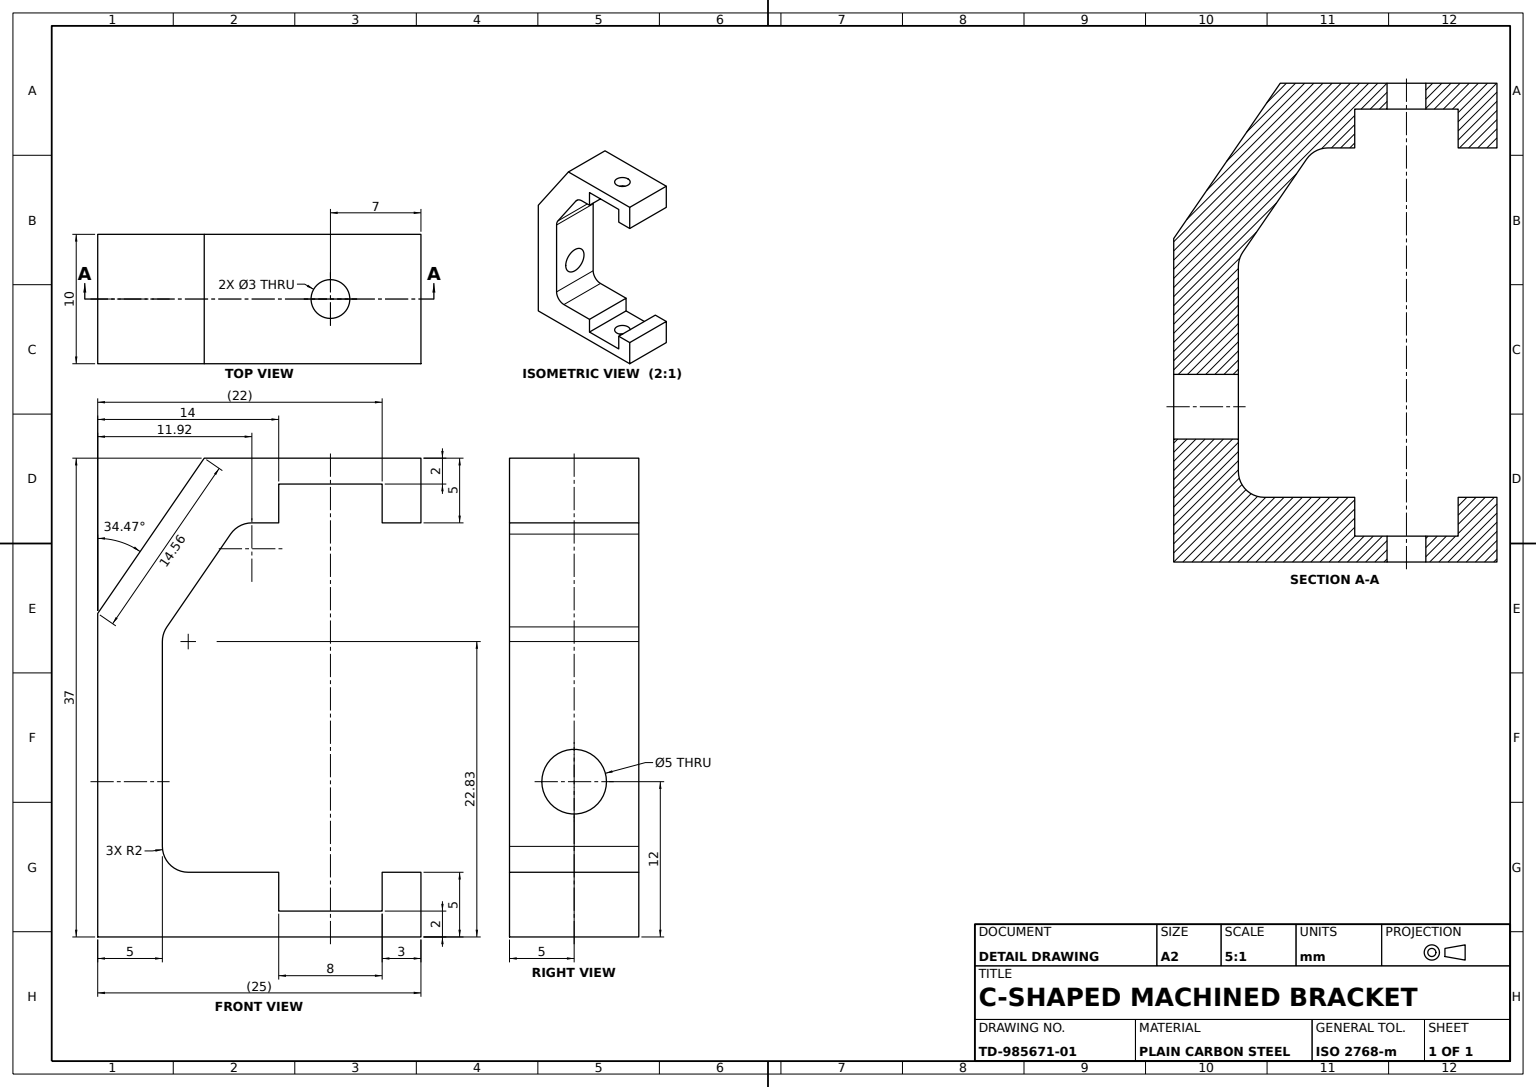
SolidWorks part; units mm, degrees
material "Plain Carbon Steel"
ref_plane "Front Plane" through (0, 0, 0) normal (0, 0, 1) x (1, 0, 0)
ref_plane "Top Plane" through (0, 0, 0) normal (0, 1, 0) x (1, 0, 0)
ref_plane "Right Plane" through (0, 0, 0) normal (1, 0, 0) x (0, 0, -1)
sketch "Bracket Profile Sketch" plane through (0, 0, 0) normal (0, 0, 1) x (1, 0, 0)
  line L0 (0, 0) -> (0, 25)
  line L1 (0, 25) -> (8.2386, 37)
  line L2 (8.2386, 37) -> (25, 37)
  line L3 (25, 37) -> (25, 32)
  line L5 (22, 32) -> (22, 35)
  line L6 (22, 35) -> (14, 35)
  line L12 (14, 5) -> (14, 2)
  line L13 (14, 2) -> (22, 2)
  line L14 (22, 2) -> (22, 5)
  line L16 (25, 5) -> (25, 0)
  line L17 (25, 0) -> (0, 0)
  line L18 (25, 5) -> (22, 5)
  line L19 (5, 7) -> (5, 22.8283)
  line L20 (5.3512, 23.9603) -> (10.2749, 31.132)
  line L21 (11.9237, 32) -> (14, 32)
  line L22 (14, 35) -> (14, 32)
  line L23 (8.2386, 32) -> (25, 32) construction
  line L24 (5, 23.4488) -> (12.3607, 34.17) construction
  line L25 (22, 32) -> (25, 32)
  line L26 (14, 5) -> (7, 5)
  line L27 (5, 5) -> (5, 23.4488) construction
  line L28 (25, 5) -> (5, 5) construction
  arc A0 (7, 5) -> (5, 7) centre (7, 7) cw
  arc A1 (5, 22.8283) -> (5.3512, 23.9603) centre (7, 22.8283) cw
  arc A2 (11.9237, 32) -> (10.2749, 31.132) centre (11.9237, 30) ccw
  dimension "D10" = 2
  dimension "D1" = 25
  dimension "D2" = 37
  dimension "D3" = 25
  dimension "D4" = 5
  dimension "D5" = 8
  dimension "D6" = 2
  dimension "D7" = 5
  dimension "D8" = 25
  dimension "D9" = 3
  dimension "D11" = 2
  dimension "D12" = 3
  dimension "D13" = 8
  dimension "D14" = 14.5559
extrude "C Bracket Body" add sketch "Bracket Profile Sketch" along normal mid plane 10
sketch "Web Hole Sketch" plane through (5, 0, 0) normal (1, 0, 0) x (0, 0, -1)
  line L0 (-5, 0) -> (5, 0) construction
  line L1 (5, 7) -> (5, 22.8283) construction
  circle A0 centre (0, 12) radius 2.5
  dimension "D1" = 5
  dimension "D2" = 12
  dimension "D3" = 5
extrude "Web Hole" cut sketch "Web Hole Sketch" against normal blind 10
sketch "Flange Hole Sketch" plane through (0, 37, 0) normal (0, 1, 0) x (1, 0, 0)
  line L1 (25, -5) -> (25, 5) construction
  line L2 (25, 5) -> (8.2386, 5) construction
  circle A0 centre (18, 0) radius 1.5
  dimension "D1" = 3
  dimension "D2" = 7
  dimension "D3" = 5
extrude "Flange Through Hole" cut sketch "Flange Hole Sketch" against normal blind 51
